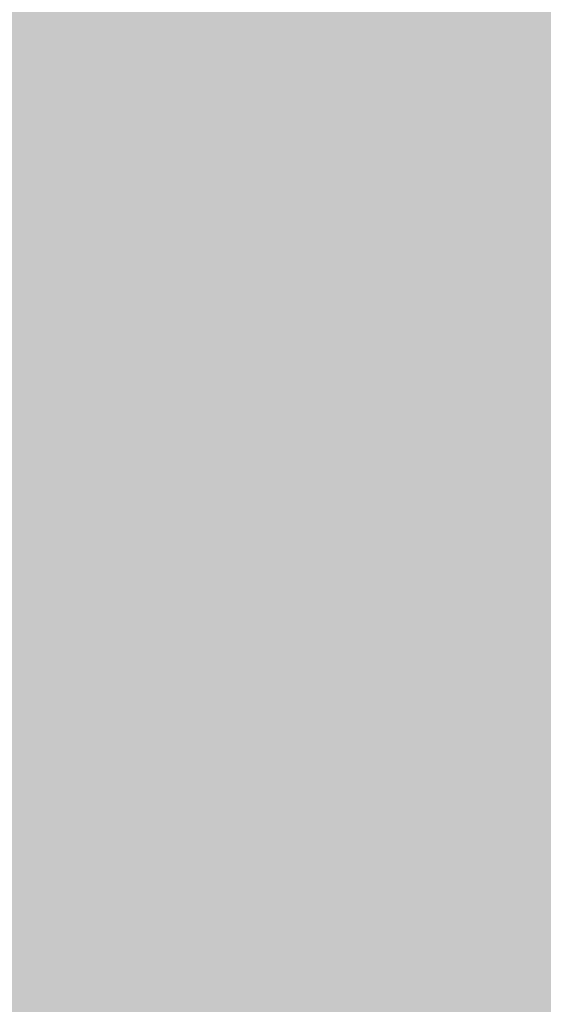
# Model space of a CAD drawing. Units: millimetres. Extents: x -22994 to 29398, y -19990 to 20176.
# Tile 83 of 135: x 227.437 to 229.428, y 79.586 to 83.328. Entities that reach past the tile are written whole.
import ezdxf
from ezdxf import colors
from ezdxf.entities.mleader import LeaderData, LeaderLine
from ezdxf.math import Vec2, Vec3

# ---------------------------------------------------------------- set-up
doc = ezdxf.new("R2010")
doc.units = ezdxf.units.MM
doc.header["$MEASUREMENT"] = 0
doc.layers.add('M-ANNO-TEXT', color=7, linetype='Continuous', lineweight=25)
doc.layers.add('M-DIMS', color=2, linetype='Continuous', lineweight=18)
doc.styles.get("Standard").update_dxf_attribs({"font": 'arial.ttf'})
doc.dimstyles.get("Standard").update_dxf_attribs({"dimtxt": 0.18, "dimasz": 10000, "dimexe": 0.18, "dimexo": 0.0625, "dimgap": 0.09, "dimtad": 0, "dimtih": 1, "dimtoh": 1, "dimdec": 0, "dimzin": 0, "dimdsep": 46, "dimtxsty": 'Standard', "dimcen": 0.09, "dimadec": 0, "dimazin": 0, "dimtfac": 1, "dimtdec": 0, "dimtofl": 0, "dimtmove": 0, "dimatfit": 3, "dimfxl": 1, "dimtolj": 1, "dimtzin": 0, "dimlwd": 30, "dimarcsym": 0})

# ---------------------------------------------------------------- blocks, each defined once
blk = doc.blocks.new('*D2')
at = {"layer": 'Defpoints', "color": 0, "transparency": 16777216}
for p in [(6.6773, 10.2713), (290.852, 10.2713), (290.852, -5.0787)]:
    blk.add_point(p, dxfattribs=at)
at = {"layer": 'M-DIMS', "color": 0, "lineweight": -2, "transparency": 16777216}
for p, q in [((6.6773, 10.2088), (6.6773, -5.2587)), ((290.852, 10.2088), (290.852, -5.2587))]:
    blk.add_line(p, q, dxfattribs=at)
at = {"layer": 'M-DIMS', "color": 0, "lineweight": 30, "transparency": 16777216}
for p, q in [((-9993.3227, -5.0787), (-19993.3227, -5.0787)), ((10290.852, -5.0787), (20290.852, -5.0787))]:
    blk.add_line(p, q, dxfattribs=at)
at = {"layer": 'M-DIMS', "color": 0, "transparency": 16777216}
for points in [[(-9993.3227, 1661.5879), (-9993.3227, -1671.7454), (6.6773, -5.0787)], [(10290.852, 1661.5879), (10290.852, -1671.7454), (290.852, -5.0787)]]:
    blk.add_solid(points, dxfattribs=at)
at = {"layer": 'M-DIMS', "color": 0, "transparency": 16777216, "insert": (148.7647, -5.0787), "char_height": 0.18, "attachment_point": 5}
blk.add_mtext('\\A1;284.2', dxfattribs=at)
blk = doc.blocks.new('*D3')
at = {"layer": 'Defpoints', "color": 0, "transparency": 16777216}
for p in [(110.2647, 204.1654), (110.2647, 176.3662), (95.8327, 127.967)]:
    blk.add_point(p, dxfattribs=at)
at = {"layer": 'M-DIMS', "color": 0, "lineweight": -2, "transparency": 16777216}
for p, q in [((95.8327, 128.0295), (95.8327, 204.3454)), ((110.2647, 176.4287), (110.2647, 204.3454))]:
    blk.add_line(p, q, dxfattribs=at)
at = {"layer": 'M-DIMS', "color": 0, "lineweight": 30, "transparency": 16777216}
for p, q in [((-9904.1673, 204.1654), (-19904.1673, 204.1654)), ((10110.2647, 204.1654), (20110.2647, 204.1654))]:
    blk.add_line(p, q, dxfattribs=at)
at = {"layer": 'M-DIMS', "color": 0, "transparency": 16777216}
for points in [[(-9904.1673, 1870.8321), (-9904.1673, -1462.5013), (95.8327, 204.1654)], [(10110.2647, 1870.8321), (10110.2647, -1462.5013), (110.2647, 204.1654)]]:
    blk.add_solid(points, dxfattribs=at)
at = {"layer": 'M-DIMS', "color": 0, "transparency": 16777216, "insert": (103.0487, 204.1654), "char_height": 0.18, "attachment_point": 5}
blk.add_mtext('\\A1;14.432', dxfattribs=at)
blk = doc.blocks.new('*D4')
at = {"layer": 'Defpoints', "color": 0, "transparency": 16777216}
for p in [(116.2647, 204.1654), (110.2647, 176.3662), (116.2647, 176.3662)]:
    blk.add_point(p, dxfattribs=at)
at = {"layer": 'M-DIMS', "color": 0, "lineweight": -2, "transparency": 16777216}
for p, q in [((110.2647, 176.4287), (110.2647, 204.3454)), ((116.2647, 176.4287), (116.2647, 204.3454))]:
    blk.add_line(p, q, dxfattribs=at)
at = {"layer": 'M-DIMS', "color": 0, "lineweight": 30, "transparency": 16777216}
for p, q in [((-9889.7353, 204.1654), (-19889.7353, 204.1654)), ((10116.2647, 204.1654), (20116.2647, 204.1654))]:
    blk.add_line(p, q, dxfattribs=at)
at = {"layer": 'M-DIMS', "color": 0, "transparency": 16777216}
for points in [[(-9889.7353, 1870.8321), (-9889.7353, -1462.5013), (110.2647, 204.1654)], [(10116.2647, 1870.8321), (10116.2647, -1462.5013), (116.2647, 204.1654)]]:
    blk.add_solid(points, dxfattribs=at)
at = {"layer": 'M-DIMS', "color": 0, "transparency": 16777216, "insert": (113.2647, 204.1654), "char_height": 0.18, "attachment_point": 5}
blk.add_mtext('\\A1;6', dxfattribs=at)
blk = doc.blocks.new('*D5')
at = {"layer": 'Defpoints', "color": 0, "transparency": 16777216}
for p in [(181.2647, 204.1654), (116.2647, 176.3662), (181.2647, 176.3662)]:
    blk.add_point(p, dxfattribs=at)
at = {"layer": 'M-DIMS', "color": 0, "lineweight": -2, "transparency": 16777216}
for p, q in [((116.2647, 176.4287), (116.2647, 204.3454)), ((181.2647, 176.4287), (181.2647, 204.3454))]:
    blk.add_line(p, q, dxfattribs=at)
at = {"layer": 'M-DIMS', "color": 0, "lineweight": 30, "transparency": 16777216}
for p, q in [((-9883.7353, 204.1654), (-19883.7353, 204.1654)), ((10181.2647, 204.1654), (20181.2647, 204.1654))]:
    blk.add_line(p, q, dxfattribs=at)
at = {"layer": 'M-DIMS', "color": 0, "transparency": 16777216}
for points in [[(-9883.7353, 1870.8321), (-9883.7353, -1462.5013), (116.2647, 204.1654)], [(10181.2647, 1870.8321), (10181.2647, -1462.5013), (181.2647, 204.1654)]]:
    blk.add_solid(points, dxfattribs=at)
at = {"layer": 'M-DIMS', "color": 0, "transparency": 16777216, "insert": (148.7647, 204.1654), "char_height": 0.18, "attachment_point": 5}
blk.add_mtext('\\A1;65', dxfattribs=at)
blk = doc.blocks.new('*D6')
at = {"layer": 'Defpoints', "color": 0, "transparency": 16777216}
for p in [(187.2647, 204.1654), (181.2647, 176.3662), (187.2647, 176.3662)]:
    blk.add_point(p, dxfattribs=at)
at = {"layer": 'M-DIMS', "color": 0, "lineweight": -2, "transparency": 16777216}
for p, q in [((181.2647, 176.4287), (181.2647, 204.3454)), ((187.2647, 176.4287), (187.2647, 204.3454))]:
    blk.add_line(p, q, dxfattribs=at)
at = {"layer": 'M-DIMS', "color": 0, "lineweight": 30, "transparency": 16777216}
for p, q in [((-9818.7353, 204.1654), (-19818.7353, 204.1654)), ((10187.2647, 204.1654), (20187.2647, 204.1654))]:
    blk.add_line(p, q, dxfattribs=at)
at = {"layer": 'M-DIMS', "color": 0, "transparency": 16777216}
for points in [[(-9818.7353, 1870.8321), (-9818.7353, -1462.5013), (181.2647, 204.1654)], [(10187.2647, 1870.8321), (10187.2647, -1462.5013), (187.2647, 204.1654)]]:
    blk.add_solid(points, dxfattribs=at)
at = {"layer": 'M-DIMS', "color": 0, "transparency": 16777216, "insert": (184.2647, 204.1654), "char_height": 0.18, "attachment_point": 5}
blk.add_mtext('\\A1;6', dxfattribs=at)
blk = doc.blocks.new('*D7')
at = {"layer": 'Defpoints', "color": 0, "transparency": 16777216}
for p in [(201.6967, 204.1654), (187.2647, 176.3662), (201.6967, 127.967)]:
    blk.add_point(p, dxfattribs=at)
at = {"layer": 'M-DIMS', "color": 0, "lineweight": -2, "transparency": 16777216}
for p, q in [((187.2647, 176.4287), (187.2647, 204.3454)), ((201.6967, 128.0295), (201.6967, 204.3454))]:
    blk.add_line(p, q, dxfattribs=at)
at = {"layer": 'M-DIMS', "color": 0, "lineweight": 30, "transparency": 16777216}
for p, q in [((-9812.7353, 204.1654), (-19812.7353, 204.1654)), ((10201.6967, 204.1654), (20201.6967, 204.1654))]:
    blk.add_line(p, q, dxfattribs=at)
at = {"layer": 'M-DIMS', "color": 0, "transparency": 16777216}
for points in [[(-9812.7353, 1870.8321), (-9812.7353, -1462.5013), (187.2647, 204.1654)], [(10201.6967, 1870.8321), (10201.6967, -1462.5013), (201.6967, 204.1654)]]:
    blk.add_solid(points, dxfattribs=at)
at = {"layer": 'M-DIMS', "color": 0, "transparency": 16777216, "insert": (194.4807, 204.1654), "char_height": 0.18, "attachment_point": 5}
blk.add_mtext('\\A1;14.432', dxfattribs=at)
blk = doc.blocks.new('*D8')
at = {"layer": 'Defpoints', "color": 0, "transparency": 16777216}
for p in [(227.6485, 204.1654), (227.6485, 146.7296), (201.6967, 127.967)]:
    blk.add_point(p, dxfattribs=at)
at = {"layer": 'M-DIMS', "color": 0, "lineweight": -2, "transparency": 16777216}
for p, q in [((201.6967, 128.0295), (201.6967, 204.3454)), ((227.6485, 146.7921), (227.6485, 204.3454))]:
    blk.add_line(p, q, dxfattribs=at)
at = {"layer": 'M-DIMS', "color": 0, "lineweight": 30, "transparency": 16777216}
for p, q in [((-9798.3033, 204.1654), (-19798.3033, 204.1654)), ((10227.6485, 204.1654), (20227.6485, 204.1654))]:
    blk.add_line(p, q, dxfattribs=at)
at = {"layer": 'M-DIMS', "color": 0, "transparency": 16777216}
for points in [[(-9798.3033, 1870.8321), (-9798.3033, -1462.5013), (201.6967, 204.1654)], [(10227.6485, 1870.8321), (10227.6485, -1462.5013), (227.6485, 204.1654)]]:
    blk.add_solid(points, dxfattribs=at)
at = {"layer": 'M-DIMS', "color": 0, "transparency": 16777216, "insert": (214.6726, 204.1654), "char_height": 0.18, "attachment_point": 5}
blk.add_mtext('\\A1;25.95', dxfattribs=at)
blk = doc.blocks.new('*D9')
at = {"layer": 'Defpoints', "color": 0, "transparency": 16777216}
for p in [(187.2647, 176.3662), (306.202, 176.3662), (290.852, 10.2713)]:
    blk.add_point(p, dxfattribs=at)
at = {"layer": 'M-DIMS', "color": 0, "lineweight": 30, "transparency": 16777216}
for p, q in [((306.202, 10176.3662), (306.202, 20176.3662)), ((306.202, -9989.7287), (306.202, -19989.7287))]:
    blk.add_line(p, q, dxfattribs=at)
at = {"layer": 'M-DIMS', "color": 0, "lineweight": -2, "transparency": 16777216}
for p, q in [((187.3272, 176.3662), (306.382, 176.3662)), ((290.9145, 10.2713), (306.382, 10.2713))]:
    blk.add_line(p, q, dxfattribs=at)
at = {"layer": 'M-DIMS', "color": 0, "transparency": 16777216}
for points in [[(-1360.4646, 10176.3662), (1972.8687, 10176.3662), (306.202, 176.3662)], [(-1360.4646, -9989.7287), (1972.8687, -9989.7287), (306.202, 10.2713)]]:
    blk.add_solid(points, dxfattribs=at)
at = {"layer": 'M-DIMS', "color": 0, "transparency": 16777216, "insert": (306.202, 93.3187), "char_height": 0.18, "attachment_point": 5}
blk.add_mtext('\\A1;166.1', dxfattribs=at)
blk = doc.blocks.new('*D10')
at = {"layer": 'Defpoints', "color": 0, "transparency": 16777216}
for p in [(125.6498, 136.0713), (133.3459, 136.0713), (133.3459, -5.0787)]:
    blk.add_point(p, dxfattribs=at)
at = {"layer": 'M-DIMS', "color": 0, "lineweight": -2, "transparency": 16777216}
for p, q in [((125.6498, 136.0088), (125.6498, -5.2587)), ((133.3459, 136.0088), (133.3459, -5.2587))]:
    blk.add_line(p, q, dxfattribs=at)
at = {"layer": 'M-DIMS', "color": 0, "lineweight": 30, "transparency": 16777216}
for p, q in [((-9874.3502, -5.0787), (-19874.3502, -5.0787)), ((10133.3459, -5.0787), (20133.3459, -5.0787))]:
    blk.add_line(p, q, dxfattribs=at)
at = {"layer": 'M-DIMS', "color": 0, "transparency": 16777216}
for points in [[(-9874.3502, 1661.5879), (-9874.3502, -1671.7454), (125.6498, -5.0787)], [(10133.3459, 1661.5879), (10133.3459, -1671.7454), (133.3459, -5.0787)]]:
    blk.add_solid(points, dxfattribs=at)
at = {"layer": 'M-DIMS', "color": 0, "transparency": 16777216, "insert": (129.4978, -5.0787), "char_height": 0.18, "attachment_point": 5}
blk.add_mtext('\\A1;7.696', dxfattribs=at)
blk = doc.blocks.new('*D11')
at = {"layer": 'Defpoints', "color": 0, "transparency": 16777216}
for p in [(133.3459, 136.0713), (135.6498, 136.0713), (135.6498, -5.0787)]:
    blk.add_point(p, dxfattribs=at)
at = {"layer": 'M-DIMS', "color": 0, "lineweight": -2, "transparency": 16777216}
for p, q in [((133.3459, 136.0088), (133.3459, -5.2587)), ((135.6498, 136.0088), (135.6498, -5.2587))]:
    blk.add_line(p, q, dxfattribs=at)
at = {"layer": 'M-DIMS', "color": 0, "lineweight": 30, "transparency": 16777216}
for p, q in [((-9866.6541, -5.0787), (-19866.6541, -5.0787)), ((10135.6498, -5.0787), (20135.6498, -5.0787))]:
    blk.add_line(p, q, dxfattribs=at)
at = {"layer": 'M-DIMS', "color": 0, "transparency": 16777216}
for points in [[(-9866.6541, 1661.5879), (-9866.6541, -1671.7454), (133.3459, -5.0787)], [(10135.6498, 1661.5879), (10135.6498, -1671.7454), (135.6498, -5.0787)]]:
    blk.add_solid(points, dxfattribs=at)
at = {"layer": 'M-DIMS', "color": 0, "transparency": 16777216, "insert": (134.4978, -5.0787), "char_height": 0.18, "attachment_point": 5}
blk.add_mtext('\\A1;2.304', dxfattribs=at)
blk = doc.blocks.new('*D12')
at = {"layer": 'Defpoints', "color": 0, "transparency": 16777216}
for p in [(135.6498, 136.0713), (145.6498, 136.0713), (145.6498, -5.0787)]:
    blk.add_point(p, dxfattribs=at)
at = {"layer": 'M-DIMS', "color": 0, "lineweight": -2, "transparency": 16777216}
for p, q in [((135.6498, 136.0088), (135.6498, -5.2587)), ((145.6498, 136.0088), (145.6498, -5.2587))]:
    blk.add_line(p, q, dxfattribs=at)
at = {"layer": 'M-DIMS', "color": 0, "lineweight": 30, "transparency": 16777216}
for p, q in [((-9864.3502, -5.0787), (-19864.3502, -5.0787)), ((10145.6498, -5.0787), (20145.6498, -5.0787))]:
    blk.add_line(p, q, dxfattribs=at)
at = {"layer": 'M-DIMS', "color": 0, "transparency": 16777216}
for points in [[(-9864.3502, 1661.5879), (-9864.3502, -1671.7454), (135.6498, -5.0787)], [(10145.6498, 1661.5879), (10145.6498, -1671.7454), (145.6498, -5.0787)]]:
    blk.add_solid(points, dxfattribs=at)
at = {"layer": 'M-DIMS', "color": 0, "transparency": 16777216, "insert": (140.6498, -5.0787), "char_height": 0.18, "attachment_point": 5}
blk.add_mtext('\\A1;10', dxfattribs=at)
blk = doc.blocks.new('*D13')
at = {"layer": 'Defpoints', "color": 0, "transparency": 16777216}
for p in [(145.6498, 136.0713), (155.6498, 136.0713), (155.6498, -5.0787)]:
    blk.add_point(p, dxfattribs=at)
at = {"layer": 'M-DIMS', "color": 0, "lineweight": -2, "transparency": 16777216}
for p, q in [((145.6498, 136.0088), (145.6498, -5.2587)), ((155.6498, 136.0088), (155.6498, -5.2587))]:
    blk.add_line(p, q, dxfattribs=at)
at = {"layer": 'M-DIMS', "color": 0, "lineweight": 30, "transparency": 16777216}
for p, q in [((-9854.3502, -5.0787), (-19854.3502, -5.0787)), ((10155.6498, -5.0787), (20155.6498, -5.0787))]:
    blk.add_line(p, q, dxfattribs=at)
at = {"layer": 'M-DIMS', "color": 0, "transparency": 16777216}
for points in [[(-9854.3502, 1661.5879), (-9854.3502, -1671.7454), (145.6498, -5.0787)], [(10155.6498, 1661.5879), (10155.6498, -1671.7454), (155.6498, -5.0787)]]:
    blk.add_solid(points, dxfattribs=at)
at = {"layer": 'M-DIMS', "color": 0, "transparency": 16777216, "insert": (150.6498, -5.0787), "char_height": 0.18, "attachment_point": 5}
blk.add_mtext('\\A1;10', dxfattribs=at)
blk = doc.blocks.new('*D14')
at = {"layer": 'Defpoints', "color": 0, "transparency": 16777216}
for p in [(155.6498, 136.0713), (165.6498, 136.0713), (165.6498, -5.0787)]:
    blk.add_point(p, dxfattribs=at)
at = {"layer": 'M-DIMS', "color": 0, "lineweight": -2, "transparency": 16777216}
for p, q in [((155.6498, 136.0088), (155.6498, -5.2587)), ((165.6498, 136.0088), (165.6498, -5.2587))]:
    blk.add_line(p, q, dxfattribs=at)
at = {"layer": 'M-DIMS', "color": 0, "lineweight": 30, "transparency": 16777216}
for p, q in [((-9844.3502, -5.0787), (-19844.3502, -5.0787)), ((10165.6498, -5.0787), (20165.6498, -5.0787))]:
    blk.add_line(p, q, dxfattribs=at)
at = {"layer": 'M-DIMS', "color": 0, "transparency": 16777216}
for points in [[(-9844.3502, 1661.5879), (-9844.3502, -1671.7454), (155.6498, -5.0787)], [(10165.6498, 1661.5879), (10165.6498, -1671.7454), (165.6498, -5.0787)]]:
    blk.add_solid(points, dxfattribs=at)
at = {"layer": 'M-DIMS', "color": 0, "transparency": 16777216, "insert": (160.6498, -5.0787), "char_height": 0.18, "attachment_point": 5}
blk.add_mtext('\\A1;10', dxfattribs=at)
blk = doc.blocks.new('*D15')
at = {"layer": 'Defpoints', "color": 0, "transparency": 16777216}
for p in [(173.3459, 154.788), (173.3459, 136.0713), (306.202, 136.0713)]:
    blk.add_point(p, dxfattribs=at)
at = {"layer": 'M-DIMS', "color": 0, "lineweight": 30, "transparency": 16777216}
for p, q in [((306.202, 10154.788), (306.202, 20154.788)), ((306.202, -9863.9287), (306.202, -19863.9287))]:
    blk.add_line(p, q, dxfattribs=at)
at = {"layer": 'M-DIMS', "color": 0, "lineweight": -2, "transparency": 16777216}
for p, q in [((173.4084, 154.788), (306.382, 154.788)), ((173.4084, 136.0713), (306.382, 136.0713))]:
    blk.add_line(p, q, dxfattribs=at)
at = {"layer": 'M-DIMS', "color": 0, "transparency": 16777216}
for points in [[(-1360.4646, 10154.788), (1972.8687, 10154.788), (306.202, 154.788)], [(-1360.4646, -9863.9287), (1972.8687, -9863.9287), (306.202, 136.0713)]]:
    blk.add_solid(points, dxfattribs=at)
at = {"layer": 'M-DIMS', "color": 0, "transparency": 16777216, "insert": (306.202, 145.4297), "char_height": 0.18, "attachment_point": 5}
blk.add_mtext('\\A1;18.717', dxfattribs=at)
blk = doc.blocks.new('*D16')
at = {"layer": 'Defpoints', "color": 0, "transparency": 16777216}
for p in [(120.1702, 204.1654), (110.4658, 48.0349), (120.1702, 48.0349)]:
    blk.add_point(p, dxfattribs=at)
at = {"layer": 'M-DIMS', "color": 0, "lineweight": -2, "transparency": 16777216}
for p, q in [((110.4658, 48.0974), (110.4658, 204.3454)), ((120.1702, 48.0974), (120.1702, 204.3454))]:
    blk.add_line(p, q, dxfattribs=at)
at = {"layer": 'M-DIMS', "color": 0, "lineweight": 30, "transparency": 16777216}
for p, q in [((-9889.5342, 204.1654), (-19889.5342, 204.1654)), ((10120.1702, 204.1654), (20120.1702, 204.1654))]:
    blk.add_line(p, q, dxfattribs=at)
at = {"layer": 'M-DIMS', "color": 0, "transparency": 16777216}
for points in [[(-9889.5342, 1870.8321), (-9889.5342, -1462.5013), (110.4658, 204.1654)], [(10120.1702, 1870.8321), (10120.1702, -1462.5013), (120.1702, 204.1654)]]:
    blk.add_solid(points, dxfattribs=at)
at = {"layer": 'M-DIMS', "color": 0, "transparency": 16777216, "insert": (115.318, 204.1654), "char_height": 0.18, "attachment_point": 5}
blk.add_mtext('\\A1;9.704', dxfattribs=at)
blk = doc.blocks.new('*D17')
at = {"layer": 'Defpoints', "color": 0, "transparency": 16777216}
for p in [(126.1702, 204.1654), (120.1702, 48.0349), (126.1702, 48.0349)]:
    blk.add_point(p, dxfattribs=at)
at = {"layer": 'M-DIMS', "color": 0, "lineweight": -2, "transparency": 16777216}
for p, q in [((120.1702, 48.0974), (120.1702, 204.3454)), ((126.1702, 48.0974), (126.1702, 204.3454))]:
    blk.add_line(p, q, dxfattribs=at)
at = {"layer": 'M-DIMS', "color": 0, "lineweight": 30, "transparency": 16777216}
for p, q in [((-9879.8298, 204.1654), (-19879.8298, 204.1654)), ((10126.1702, 204.1654), (20126.1702, 204.1654))]:
    blk.add_line(p, q, dxfattribs=at)
at = {"layer": 'M-DIMS', "color": 0, "transparency": 16777216}
for points in [[(-9879.8298, 1870.8321), (-9879.8298, -1462.5013), (120.1702, 204.1654)], [(10126.1702, 1870.8321), (10126.1702, -1462.5013), (126.1702, 204.1654)]]:
    blk.add_solid(points, dxfattribs=at)
at = {"layer": 'M-DIMS', "color": 0, "transparency": 16777216, "insert": (123.1702, 204.1654), "char_height": 0.18, "attachment_point": 5}
blk.add_mtext('\\A1;6', dxfattribs=at)
blk = doc.blocks.new('*D18')
at = {"layer": 'Defpoints', "color": 0, "transparency": 16777216}
for p in [(132.1702, 204.1654), (126.1702, 48.0349), (132.1702, 48.0349)]:
    blk.add_point(p, dxfattribs=at)
at = {"layer": 'M-DIMS', "color": 0, "lineweight": -2, "transparency": 16777216}
for p, q in [((126.1702, 48.0974), (126.1702, 204.3454)), ((132.1702, 48.0974), (132.1702, 204.3454))]:
    blk.add_line(p, q, dxfattribs=at)
at = {"layer": 'M-DIMS', "color": 0, "lineweight": 30, "transparency": 16777216}
for p, q in [((-9873.8298, 204.1654), (-19873.8298, 204.1654)), ((10132.1702, 204.1654), (20132.1702, 204.1654))]:
    blk.add_line(p, q, dxfattribs=at)
at = {"layer": 'M-DIMS', "color": 0, "transparency": 16777216}
for points in [[(-9873.8298, 1870.8321), (-9873.8298, -1462.5013), (126.1702, 204.1654)], [(10132.1702, 1870.8321), (10132.1702, -1462.5013), (132.1702, 204.1654)]]:
    blk.add_solid(points, dxfattribs=at)
at = {"layer": 'M-DIMS', "color": 0, "transparency": 16777216, "insert": (129.1702, 204.1654), "char_height": 0.18, "attachment_point": 5}
blk.add_mtext('\\A1;6', dxfattribs=at)
blk = doc.blocks.new('*D19')
at = {"layer": 'Defpoints', "color": 0, "transparency": 16777216}
for p in [(138.1702, 204.1654), (132.1702, 48.0349), (138.1702, 48.0349)]:
    blk.add_point(p, dxfattribs=at)
at = {"layer": 'M-DIMS', "color": 0, "lineweight": -2, "transparency": 16777216}
for p, q in [((132.1702, 48.0974), (132.1702, 204.3454)), ((138.1702, 48.0974), (138.1702, 204.3454))]:
    blk.add_line(p, q, dxfattribs=at)
at = {"layer": 'M-DIMS', "color": 0, "lineweight": 30, "transparency": 16777216}
for p, q in [((-9867.8298, 204.1654), (-19867.8298, 204.1654)), ((10138.1702, 204.1654), (20138.1702, 204.1654))]:
    blk.add_line(p, q, dxfattribs=at)
at = {"layer": 'M-DIMS', "color": 0, "transparency": 16777216}
for points in [[(-9867.8298, 1870.8321), (-9867.8298, -1462.5013), (132.1702, 204.1654)], [(10138.1702, 1870.8321), (10138.1702, -1462.5013), (138.1702, 204.1654)]]:
    blk.add_solid(points, dxfattribs=at)
at = {"layer": 'M-DIMS', "color": 0, "transparency": 16777216, "insert": (135.1702, 204.1654), "char_height": 0.18, "attachment_point": 5}
blk.add_mtext('\\A1;6', dxfattribs=at)
blk = doc.blocks.new('*D20')
at = {"layer": 'Defpoints', "color": 0, "transparency": 16777216}
for p in [(144.1702, 204.1654), (138.1702, 48.0349), (144.1702, 48.0349)]:
    blk.add_point(p, dxfattribs=at)
at = {"layer": 'M-DIMS', "color": 0, "lineweight": -2, "transparency": 16777216}
for p, q in [((138.1702, 48.0974), (138.1702, 204.3454)), ((144.1702, 48.0974), (144.1702, 204.3454))]:
    blk.add_line(p, q, dxfattribs=at)
at = {"layer": 'M-DIMS', "color": 0, "lineweight": 30, "transparency": 16777216}
for p, q in [((-9861.8298, 204.1654), (-19861.8298, 204.1654)), ((10144.1702, 204.1654), (20144.1702, 204.1654))]:
    blk.add_line(p, q, dxfattribs=at)
at = {"layer": 'M-DIMS', "color": 0, "transparency": 16777216}
for points in [[(-9861.8298, 1870.8321), (-9861.8298, -1462.5013), (138.1702, 204.1654)], [(10144.1702, 1870.8321), (10144.1702, -1462.5013), (144.1702, 204.1654)]]:
    blk.add_solid(points, dxfattribs=at)
at = {"layer": 'M-DIMS', "color": 0, "transparency": 16777216, "insert": (141.1702, 204.1654), "char_height": 0.18, "attachment_point": 5}
blk.add_mtext('\\A1;6', dxfattribs=at)
blk = doc.blocks.new('*D21')
at = {"layer": 'Defpoints', "color": 0, "transparency": 16777216}
for p in [(149.1157, 204.1654), (144.1702, 48.0349), (149.1157, 48.0349)]:
    blk.add_point(p, dxfattribs=at)
at = {"layer": 'M-DIMS', "color": 0, "lineweight": -2, "transparency": 16777216}
for p, q in [((144.1702, 48.0974), (144.1702, 204.3454)), ((149.1157, 48.0974), (149.1157, 204.3454))]:
    blk.add_line(p, q, dxfattribs=at)
at = {"layer": 'M-DIMS', "color": 0, "lineweight": 30, "transparency": 16777216}
for p, q in [((-9855.8298, 204.1654), (-19855.8298, 204.1654)), ((10149.1157, 204.1654), (20149.1157, 204.1654))]:
    blk.add_line(p, q, dxfattribs=at)
at = {"layer": 'M-DIMS', "color": 0, "transparency": 16777216}
for points in [[(-9855.8298, 1870.8321), (-9855.8298, -1462.5013), (144.1702, 204.1654)], [(10149.1157, 1870.8321), (10149.1157, -1462.5013), (149.1157, 204.1654)]]:
    blk.add_solid(points, dxfattribs=at)
at = {"layer": 'M-DIMS', "color": 0, "transparency": 16777216, "insert": (146.6429, 204.1654), "char_height": 0.18, "attachment_point": 5}
blk.add_mtext('\\A1;4.945', dxfattribs=at)
blk = doc.blocks.new('*D22')
at = {"layer": 'Defpoints', "color": 0, "transparency": 16777216}
for p in [(149.1157, 30.9895), (155.1157, 30.9895), (155.1157, -5.0787)]:
    blk.add_point(p, dxfattribs=at)
at = {"layer": 'M-DIMS', "color": 0, "lineweight": -2, "transparency": 16777216}
for p, q in [((149.1157, 30.927), (149.1157, -5.2587)), ((155.1157, 30.927), (155.1157, -5.2587))]:
    blk.add_line(p, q, dxfattribs=at)
at = {"layer": 'M-DIMS', "color": 0, "lineweight": 30, "transparency": 16777216}
for p, q in [((-9850.8843, -5.0787), (-19850.8843, -5.0787)), ((10155.1157, -5.0787), (20155.1157, -5.0787))]:
    blk.add_line(p, q, dxfattribs=at)
at = {"layer": 'M-DIMS', "color": 0, "transparency": 16777216}
for points in [[(-9850.8843, 1661.5879), (-9850.8843, -1671.7454), (149.1157, -5.0787)], [(10155.1157, 1661.5879), (10155.1157, -1671.7454), (155.1157, -5.0787)]]:
    blk.add_solid(points, dxfattribs=at)
at = {"layer": 'M-DIMS', "color": 0, "transparency": 16777216, "insert": (152.1157, -5.0787), "char_height": 0.18, "attachment_point": 5}
blk.add_mtext('\\A1;6', dxfattribs=at)
blk = doc.blocks.new('*D23')
at = {"layer": 'Defpoints', "color": 0, "transparency": 16777216}
for p in [(155.1157, 30.9895), (161.1157, 30.9895), (161.1157, -5.0787)]:
    blk.add_point(p, dxfattribs=at)
at = {"layer": 'M-DIMS', "color": 0, "lineweight": -2, "transparency": 16777216}
for p, q in [((155.1157, 30.927), (155.1157, -5.2587)), ((161.1157, 30.927), (161.1157, -5.2587))]:
    blk.add_line(p, q, dxfattribs=at)
at = {"layer": 'M-DIMS', "color": 0, "lineweight": 30, "transparency": 16777216}
for p, q in [((-9844.8843, -5.0787), (-19844.8843, -5.0787)), ((10161.1157, -5.0787), (20161.1157, -5.0787))]:
    blk.add_line(p, q, dxfattribs=at)
at = {"layer": 'M-DIMS', "color": 0, "transparency": 16777216}
for points in [[(-9844.8843, 1661.5879), (-9844.8843, -1671.7454), (155.1157, -5.0787)], [(10161.1157, 1661.5879), (10161.1157, -1671.7454), (161.1157, -5.0787)]]:
    blk.add_solid(points, dxfattribs=at)
at = {"layer": 'M-DIMS', "color": 0, "transparency": 16777216, "insert": (158.1157, -5.0787), "char_height": 0.18, "attachment_point": 5}
blk.add_mtext('\\A1;6', dxfattribs=at)
blk = doc.blocks.new('*D24')
at = {"layer": 'Defpoints', "color": 0, "transparency": 16777216}
for p in [(161.1157, 30.9895), (166.4387, 30.9895), (166.4387, -5.0787)]:
    blk.add_point(p, dxfattribs=at)
at = {"layer": 'M-DIMS', "color": 0, "lineweight": -2, "transparency": 16777216}
for p, q in [((161.1157, 30.927), (161.1157, -5.2587)), ((166.4387, 30.927), (166.4387, -5.2587))]:
    blk.add_line(p, q, dxfattribs=at)
at = {"layer": 'M-DIMS', "color": 0, "lineweight": 30, "transparency": 16777216}
for p, q in [((-9838.8843, -5.0787), (-19838.8843, -5.0787)), ((10166.4387, -5.0787), (20166.4387, -5.0787))]:
    blk.add_line(p, q, dxfattribs=at)
at = {"layer": 'M-DIMS', "color": 0, "transparency": 16777216}
for points in [[(-9838.8843, 1661.5879), (-9838.8843, -1671.7454), (161.1157, -5.0787)], [(10166.4387, 1661.5879), (10166.4387, -1671.7454), (166.4387, -5.0787)]]:
    blk.add_solid(points, dxfattribs=at)
at = {"layer": 'M-DIMS', "color": 0, "transparency": 16777216, "insert": (163.7772, -5.0787), "char_height": 0.18, "attachment_point": 5}
blk.add_mtext('\\A1;5.323', dxfattribs=at)
blk = doc.blocks.new('*D25')
at = {"layer": 'Defpoints', "color": 0, "transparency": 16777216}
for p in [(166.4387, 30.9895), (172.4387, 30.9895), (172.4387, -5.0787)]:
    blk.add_point(p, dxfattribs=at)
at = {"layer": 'M-DIMS', "color": 0, "lineweight": -2, "transparency": 16777216}
for p, q in [((166.4387, 30.927), (166.4387, -5.2587)), ((172.4387, 30.927), (172.4387, -5.2587))]:
    blk.add_line(p, q, dxfattribs=at)
at = {"layer": 'M-DIMS', "color": 0, "lineweight": 30, "transparency": 16777216}
for p, q in [((-9833.5613, -5.0787), (-19833.5613, -5.0787)), ((10172.4387, -5.0787), (20172.4387, -5.0787))]:
    blk.add_line(p, q, dxfattribs=at)
at = {"layer": 'M-DIMS', "color": 0, "transparency": 16777216}
for points in [[(-9833.5613, 1661.5879), (-9833.5613, -1671.7454), (166.4387, -5.0787)], [(10172.4387, 1661.5879), (10172.4387, -1671.7454), (172.4387, -5.0787)]]:
    blk.add_solid(points, dxfattribs=at)
at = {"layer": 'M-DIMS', "color": 0, "transparency": 16777216, "insert": (169.4387, -5.0787), "char_height": 0.18, "attachment_point": 5}
blk.add_mtext('\\A1;6', dxfattribs=at)
blk = doc.blocks.new('*D26')
at = {"layer": 'Defpoints', "color": 0, "transparency": 16777216}
for p in [(172.4387, 30.9895), (178.4387, 30.9895), (178.4387, -5.0787)]:
    blk.add_point(p, dxfattribs=at)
at = {"layer": 'M-DIMS', "color": 0, "lineweight": -2, "transparency": 16777216}
for p, q in [((172.4387, 30.927), (172.4387, -5.2587)), ((178.4387, 30.927), (178.4387, -5.2587))]:
    blk.add_line(p, q, dxfattribs=at)
at = {"layer": 'M-DIMS', "color": 0, "lineweight": 30, "transparency": 16777216}
for p, q in [((-9827.5613, -5.0787), (-19827.5613, -5.0787)), ((10178.4387, -5.0787), (20178.4387, -5.0787))]:
    blk.add_line(p, q, dxfattribs=at)
at = {"layer": 'M-DIMS', "color": 0, "transparency": 16777216}
for points in [[(-9827.5613, 1661.5879), (-9827.5613, -1671.7454), (172.4387, -5.0787)], [(10178.4387, 1661.5879), (10178.4387, -1671.7454), (178.4387, -5.0787)]]:
    blk.add_solid(points, dxfattribs=at)
at = {"layer": 'M-DIMS', "color": 0, "transparency": 16777216, "insert": (175.4387, -5.0787), "char_height": 0.18, "attachment_point": 5}
blk.add_mtext('\\A1;6', dxfattribs=at)
blk = doc.blocks.new('*D27')
at = {"layer": 'Defpoints', "color": 0, "transparency": 16777216}
for p in [(178.4387, 30.9895), (188.1175, 30.9895), (188.1175, -5.0787)]:
    blk.add_point(p, dxfattribs=at)
at = {"layer": 'M-DIMS', "color": 0, "lineweight": -2, "transparency": 16777216}
for p, q in [((178.4387, 30.927), (178.4387, -5.2587)), ((188.1175, 30.927), (188.1175, -5.2587))]:
    blk.add_line(p, q, dxfattribs=at)
at = {"layer": 'M-DIMS', "color": 0, "lineweight": 30, "transparency": 16777216}
for p, q in [((-9821.5613, -5.0787), (-19821.5613, -5.0787)), ((10188.1175, -5.0787), (20188.1175, -5.0787))]:
    blk.add_line(p, q, dxfattribs=at)
at = {"layer": 'M-DIMS', "color": 0, "transparency": 16777216}
for points in [[(-9821.5613, 1661.5879), (-9821.5613, -1671.7454), (178.4387, -5.0787)], [(10188.1175, 1661.5879), (10188.1175, -1671.7454), (188.1175, -5.0787)]]:
    blk.add_solid(points, dxfattribs=at)
at = {"layer": 'M-DIMS', "color": 0, "transparency": 16777216, "insert": (183.2781, -5.0787), "char_height": 0.18, "attachment_point": 5}
blk.add_mtext('\\A1;9.679', dxfattribs=at)
blk = doc.blocks.new('*D28')
at = {"layer": 'Defpoints', "color": 0, "transparency": 16777216}
for p in [(188.1175, 48.0349), (306.202, 48.0349), (188.1175, 30.9895)]:
    blk.add_point(p, dxfattribs=at)
at = {"layer": 'M-DIMS', "color": 0, "lineweight": 30, "transparency": 16777216}
for p, q in [((306.202, 10048.0349), (306.202, 20048.0349)), ((306.202, -9969.0105), (306.202, -19969.0105))]:
    blk.add_line(p, q, dxfattribs=at)
at = {"layer": 'M-DIMS', "color": 0, "lineweight": -2, "transparency": 16777216}
for p, q in [((188.18, 48.0349), (306.382, 48.0349)), ((188.18, 30.9895), (306.382, 30.9895))]:
    blk.add_line(p, q, dxfattribs=at)
at = {"layer": 'M-DIMS', "color": 0, "transparency": 16777216}
for points in [[(-1360.4646, 10048.0349), (1972.8687, 10048.0349), (306.202, 48.0349)], [(-1360.4646, -9969.0105), (1972.8687, -9969.0105), (306.202, 30.9895)]]:
    blk.add_solid(points, dxfattribs=at)
at = {"layer": 'M-DIMS', "color": 0, "transparency": 16777216, "insert": (306.202, 39.5122), "char_height": 0.18, "attachment_point": 5}
blk.add_mtext('\\A1;17.045', dxfattribs=at)
blk = doc.blocks.new('*D29')
at = {"layer": 'Defpoints', "color": 0, "transparency": 16777216}
for p in [(36.8006, 80.045), (64.0296, 80.045)]:
    blk.add_point(p, dxfattribs=at)
at = {"layer": 'M-DIMS', "color": 0, "lineweight": -2, "transparency": 16777216}
for p, q in [((50.4151, 79.955), (50.4151, 80.135)), ((50.3251, 80.045), (50.5051, 80.045))]:
    blk.add_line(p, q, dxfattribs=at)
at = {"layer": 'M-DIMS', "color": 0, "lineweight": 30, "transparency": 16777216}
blk.add_line((20064.0296, 80.0303), (10064.0296, 80.0377), dxfattribs=at)
at = {"layer": 'M-DIMS', "color": 0, "transparency": 16777216}
blk.add_solid([(10064.0309, 1746.7043), (10064.0284, -1586.629), (64.0296, 80.045)], dxfattribs=at)
at = {"layer": 'M-DIMS', "color": 0, "transparency": 16777216, "insert": (20064.5213, 80.0303), "char_height": 0.18, "attachment_point": 5}
blk.add_mtext('\\A1;∅27.23', dxfattribs=at)
blk = doc.blocks.new('*D30')
at = {"layer": 'Defpoints', "color": 0, "transparency": 16777216}
for p in [(216.3148, 146.7291), (238.9821, 146.73)]:
    blk.add_point(p, dxfattribs=at)
at = {"layer": 'M-DIMS', "color": 0, "lineweight": 30, "transparency": 16777216}
blk.add_line((20238.9821, 147.4959), (10238.9821, 147.1129), dxfattribs=at)
at = {"layer": 'M-DIMS', "color": 0, "lineweight": -2, "transparency": 16777216}
for p, q in [((227.6485, 146.6396), (227.6485, 146.8196)), ((227.5585, 146.7296), (227.7385, 146.7296))]:
    blk.add_line(p, q, dxfattribs=at)
at = {"layer": 'M-DIMS', "color": 0, "transparency": 16777216}
blk.add_solid([(10238.9183, 1813.7796), (10239.0459, -1519.5537), (238.9821, 146.73)], dxfattribs=at)
at = {"layer": 'M-DIMS', "color": 0, "transparency": 16777216, "insert": (20239.5436, 147.4959), "char_height": 0.18, "attachment_point": 5}
blk.add_mtext('\\A1;∅22.667', dxfattribs=at)
blk = doc.blocks.new('*D31')
at = {"layer": 'Defpoints', "color": 0, "transparency": 16777216}
for p in [(223.1641, 146.7291), (232.1328, 146.73)]:
    blk.add_point(p, dxfattribs=at)
at = {"layer": 'M-DIMS', "color": 0, "lineweight": 30, "transparency": 16777216}
blk.add_line((20232.1327, 148.6656), (10232.1328, 147.6978), dxfattribs=at)
at = {"layer": 'M-DIMS', "color": 0, "lineweight": -2, "transparency": 16777216}
for p, q in [((227.6485, 146.6396), (227.6485, 146.8196)), ((227.5585, 146.7296), (227.7385, 146.7296))]:
    blk.add_line(p, q, dxfattribs=at)
at = {"layer": 'M-DIMS', "color": 0, "transparency": 16777216}
blk.add_solid([(10231.9715, 1814.3645), (10232.2941, -1518.9688), (232.1328, 146.73)], dxfattribs=at)
at = {"layer": 'M-DIMS', "color": 0, "transparency": 16777216, "insert": (20232.6245, 148.6656), "char_height": 0.18, "attachment_point": 5}
blk.add_mtext('\\A1;∅8.969', dxfattribs=at)
blk = doc.blocks.new('*D36')
at = {"layer": 'Defpoints', "color": 0, "transparency": 16777216}
for p in [(46.39, 31.3035), (46.3875, 26.5934)]:
    blk.add_point(p, dxfattribs=at)
at = {"layer": 'M-DIMS', "color": 0, "lineweight": 30, "transparency": 16777216}
for p, q in [((57.1499, 20031.3006), (51.77, 10031.302)), ((10057.1499, 20031.3006), (57.1499, 20031.3006))]:
    blk.add_line(p, q, dxfattribs=at)
at = {"layer": 'M-DIMS', "color": 0, "lineweight": -2, "transparency": 16777216}
for p, q in [((46.3887, 28.8585), (46.3887, 29.0385)), ((46.2987, 28.9485), (46.4787, 28.9485))]:
    blk.add_line(p, q, dxfattribs=at)
at = {"layer": 'M-DIMS', "color": 0, "transparency": 16777216}
blk.add_solid([(-1614.8965, 10032.1987), (1718.4364, 10030.4054), (46.39, 31.3035)], dxfattribs=at)
at = {"layer": 'M-DIMS', "color": 0, "transparency": 16777216, "insert": (10057.5542, 20031.3006), "char_height": 0.18, "attachment_point": 5}
blk.add_mtext('\\A1;∅4.71', dxfattribs=at)
blk = doc.blocks.new('*D37')
at = {"layer": 'Defpoints', "color": 0, "transparency": 16777216}
for p in [(54.8343, 118.6145), (59.4936, 118.614)]:
    blk.add_point(p, dxfattribs=at)
at = {"layer": 'M-DIMS', "color": 0, "lineweight": -2, "transparency": 16777216}
for p, q in [((57.1639, 118.5243), (57.1639, 118.7043)), ((57.0739, 118.6143), (57.2539, 118.6143))]:
    blk.add_line(p, q, dxfattribs=at)
at = {"layer": 'M-DIMS', "color": 0, "lineweight": 30, "transparency": 16777216}
blk.add_line((20059.4934, 116.2531), (10059.4935, 117.4336), dxfattribs=at)
at = {"layer": 'M-DIMS', "color": 0, "transparency": 16777216}
blk.add_solid([(10059.6902, 1784.1002), (10059.2968, -1549.2331), (59.4936, 118.614)], dxfattribs=at)
at = {"layer": 'M-DIMS', "color": 0, "transparency": 16777216, "insert": (20059.9852, 116.2531), "char_height": 0.18, "attachment_point": 5}
blk.add_mtext('\\A1;∅4.659', dxfattribs=at)

msp = doc.modelspace()

# ---------------------------------------------------------------- dimensions: what is measured, and where the dimension line sits
at = {"layer": 'M-DIMS'}
for base, p1, p2, override, picture, middle in [((306.202, 176.3662), (290.852, 10.2713), (187.2647, 176.3662), {"dimdec": 1, "dimlfac": 1, "dimrnd": 0, "dimzin": 0, "dimdsep": 46, "dimlunit": 2}, '*D9', (306.202, 93.3187)), ((306.202, 136.0713), (173.3459, 154.788), (173.3459, 136.0713), {"dimdec": 3, "dimlfac": 1, "dimrnd": 0, "dimzin": 0, "dimdsep": 46, "dimlunit": 2}, '*D15', (306.202, 145.4297)), ((306.202, 48.0349), (188.1175, 30.9895), (188.1175, 48.0349), {"dimdec": 3, "dimlfac": 1, "dimrnd": 0, "dimzin": 0, "dimdsep": 46, "dimlunit": 2}, '*D28', (306.202, 39.5122))]:
    dim = msp.add_linear_dim(base=base, p1=p1, p2=p2, angle=90, dimstyle='Standard', override=override, dxfattribs=at)
    dim.commit()
    dim.dimension.update_dxf_attribs({"geometry": picture, "text_midpoint": middle})
for p1, p2, override, picture, middle in [((46.3875, 26.5934), (46.39, 31.3035), {"dimdec": 2, "dimlfac": 1, "dimrnd": 0, "dimzin": 0, "dimdsep": 46, "dimlunit": 2}, '*D36', (10057.5542, 20031.3006)), ((223.1641, 146.7291), (232.1328, 146.73), {"dimdec": 3, "dimlfac": 1, "dimrnd": 0, "dimzin": 0, "dimdsep": 46, "dimlunit": 2}, '*D31', (20232.1327, 148.6656)), ((216.3148, 146.7291), (238.9821, 146.73), {"dimdec": 3, "dimlfac": 1, "dimrnd": 0, "dimzin": 0, "dimdsep": 46, "dimlunit": 2}, '*D30', (20238.9821, 147.4959))]:
    dim = msp.add_diameter_dim_2p(p1=p1, p2=p2, dimstyle='Standard', override=override, dxfattribs=at)
    dim.commit()
    dim.dimension.update_dxf_attribs({"geometry": picture, "text_midpoint": middle, "dimtype": 163})
for base, p1, p2, override, picture, middle in [((110.2647, 204.1654), (95.8327, 127.967), (110.2647, 176.3662), {"dimdec": 3, "dimlfac": 1, "dimrnd": 0, "dimzin": 0, "dimdsep": 46, "dimlunit": 2}, '*D3', (103.0487, 204.1654)), ((116.2647, 204.1654), (110.2647, 176.3662), (116.2647, 176.3662), {"dimdec": 0, "dimlfac": 1, "dimrnd": 0, "dimzin": 0, "dimdsep": 46, "dimlunit": 2}, '*D4', (113.2647, 204.1654)), ((120.1702, 204.1654), (110.4658, 48.0349), (120.1702, 48.0349), {"dimdec": 3, "dimlfac": 1, "dimrnd": 0, "dimzin": 0, "dimdsep": 46, "dimlunit": 2}, '*D16', (115.318, 204.1654)), ((181.2647, 204.1654), (116.2647, 176.3662), (181.2647, 176.3662), {"dimdec": 0, "dimlfac": 1, "dimrnd": 0, "dimzin": 0, "dimdsep": 46, "dimlunit": 2}, '*D5', (148.7647, 204.1654)), ((126.1702, 204.1654), (120.1702, 48.0349), (126.1702, 48.0349), {"dimdec": 0, "dimlfac": 1, "dimrnd": 0, "dimzin": 0, "dimdsep": 46, "dimlunit": 2}, '*D17', (123.1702, 204.1654)), ((132.1702, 204.1654), (126.1702, 48.0349), (132.1702, 48.0349), {"dimdec": 0, "dimlfac": 1, "dimrnd": 0, "dimzin": 0, "dimdsep": 46, "dimlunit": 2}, '*D18', (129.1702, 204.1654)), ((138.1702, 204.1654), (132.1702, 48.0349), (138.1702, 48.0349), {"dimdec": 0, "dimlfac": 1, "dimrnd": 0, "dimzin": 0, "dimdsep": 46, "dimlunit": 2}, '*D19', (135.1702, 204.1654)), ((144.1702, 204.1654), (138.1702, 48.0349), (144.1702, 48.0349), {"dimdec": 0, "dimlfac": 1, "dimrnd": 0, "dimzin": 0, "dimdsep": 46, "dimlunit": 2}, '*D20', (141.1702, 204.1654)), ((149.11567, 204.16539), (144.17023, 48.03494), (149.11567, 48.03494), {"dimdec": 3, "dimlfac": 1, "dimrnd": 0, "dimzin": 0, "dimdsep": 46, "dimlunit": 2}, '*D21', (146.64295, 204.16539)), ((187.2647, 204.1654), (181.2647, 176.3662), (187.2647, 176.3662), {"dimdec": 0, "dimlfac": 1, "dimrnd": 0, "dimzin": 0, "dimdsep": 46, "dimlunit": 2}, '*D6', (184.2647, 204.1654)), ((201.6967, 204.1654), (187.2647, 176.3662), (201.6967, 127.967), {"dimdec": 3, "dimlfac": 1, "dimrnd": 0, "dimzin": 0, "dimdsep": 46, "dimlunit": 2}, '*D7', (194.4807, 204.1654)), ((227.6485, 204.1654), (201.6967, 127.967), (227.6485, 146.7296), {"dimdec": 2, "dimlfac": 1, "dimrnd": 0, "dimzin": 0, "dimdsep": 46, "dimlunit": 2}, '*D8', (214.6726, 204.1654)), ((290.852, -5.0787), (6.6773, 10.2713), (290.852, 10.2713), {"dimdec": 1, "dimlfac": 1, "dimrnd": 0, "dimzin": 0, "dimdsep": 46, "dimlunit": 2}, '*D2', (148.7647, -5.0787)), ((133.3459, -5.0787), (125.6498, 136.0713), (133.3459, 136.0713), {"dimdec": 3, "dimlfac": 1, "dimrnd": 0, "dimzin": 0, "dimdsep": 46, "dimlunit": 2}, '*D10', (129.4978, -5.0787)), ((135.6498, -5.0787), (133.3459, 136.0713), (135.6498, 136.0713), {"dimdec": 3, "dimlfac": 1, "dimrnd": 0, "dimzin": 0, "dimdsep": 46, "dimlunit": 2}, '*D11', (134.4978, -5.0787)), ((145.6498, -5.0787), (135.6498, 136.0713), (145.6498, 136.0713), {"dimdec": 0, "dimlfac": 1, "dimrnd": 0, "dimzin": 0, "dimdsep": 46, "dimlunit": 2}, '*D12', (140.6498, -5.0787)), ((155.6498, -5.0787), (145.6498, 136.0713), (155.6498, 136.0713), {"dimdec": 0, "dimlfac": 1, "dimrnd": 0, "dimzin": 0, "dimdsep": 46, "dimlunit": 2}, '*D13', (150.6498, -5.0787)), ((155.1157, -5.0787), (149.1157, 30.9895), (155.1157, 30.9895), {"dimdec": 0, "dimlfac": 1, "dimrnd": 0, "dimzin": 0, "dimdsep": 46, "dimlunit": 2}, '*D22', (152.1157, -5.0787)), ((161.1157, -5.0787), (155.1157, 30.9895), (161.1157, 30.9895), {"dimdec": 0, "dimlfac": 1, "dimrnd": 0, "dimzin": 0, "dimdsep": 46, "dimlunit": 2}, '*D23', (158.1157, -5.0787)), ((165.6498, -5.0787), (155.6498, 136.0713), (165.6498, 136.0713), {"dimdec": 0, "dimlfac": 1, "dimrnd": 0, "dimzin": 0, "dimdsep": 46, "dimlunit": 2}, '*D14', (160.6498, -5.0787)), ((166.4387, -5.0787), (161.1157, 30.9895), (166.4387, 30.9895), {"dimdec": 3, "dimlfac": 1, "dimrnd": 0, "dimzin": 0, "dimdsep": 46, "dimlunit": 2}, '*D24', (163.7772, -5.0787)), ((172.4387, -5.0787), (166.4387, 30.9895), (172.4387, 30.9895), {"dimdec": 0, "dimlfac": 1, "dimrnd": 0, "dimzin": 0, "dimdsep": 46, "dimlunit": 2}, '*D25', (169.4387, -5.0787)), ((178.4387, -5.0787), (172.4387, 30.9895), (178.4387, 30.9895), {"dimdec": 0, "dimlfac": 1, "dimrnd": 0, "dimzin": 0, "dimdsep": 46, "dimlunit": 2}, '*D26', (175.4387, -5.0787)), ((188.1175, -5.0787), (178.4387, 30.9895), (188.1175, 30.9895), {"dimdec": 3, "dimlfac": 1, "dimrnd": 0, "dimzin": 0, "dimdsep": 46, "dimlunit": 2}, '*D27', (183.2781, -5.0787))]:
    dim = msp.add_linear_dim(base=base, p1=p1, p2=p2, dimstyle='Standard', override=override, dxfattribs=at)
    dim.commit()
    dim.dimension.update_dxf_attribs({"geometry": picture, "text_midpoint": middle})
for p1, p2, override, picture, middle in [((54.8343, 118.6145), (59.4936, 118.614), {"dimdec": 3, "dimlfac": 1, "dimrnd": 0, "dimzin": 0, "dimdsep": 46, "dimlunit": 2}, '*D37', (20059.4934, 116.2531)), ((36.8006, 80.045), (64.0296, 80.045), {"dimdec": 2, "dimlfac": 1, "dimrnd": 0, "dimzin": 0, "dimdsep": 46, "dimlunit": 2}, '*D29', (20064.0296, 80.0303))]:
    dim = msp.add_diameter_dim_2p(p1=p1, p2=p2, dimstyle='Standard', override=override, dxfattribs=at)
    dim.commit()
    dim.dimension.update_dxf_attribs({"geometry": picture, "text_midpoint": middle})

# ---------------------------------------------------------------- leaders
at = {"layer": 'M-ANNO-TEXT'}
ml = msp.add_multileader_mtext('Standard', dxfattribs=at)
ml.set_content('combustion chamber', color=256)
ml.set_leader_properties()
ml.build(insert=Vec2(0, 0))
ml.multileader.update_dxf_attribs({"dogleg_length": 0.36, "arrow_head_size": 200})
ctx = ml.context
ctx.base_point, ctx.char_height, ctx.arrow_head_size, ctx.landing_gap_size, ctx.plane_origin = Vec3(215.7321, 57.9149), 3, 200, 0.09, Vec3(189.1175, 57.9149)
notes = []
notes.append((ctx, [(0, (1, 1, 0), (215.3721, 57.9149), (1, 0), 0.36, [(0, [(189.1175, 57.9149)], 0, [])])]))
ctx.mtext.insert, ctx.mtext.flow_direction = Vec3(215.8221, 59.4394), 5
for ctx, leaders in notes:
    for number, flags, end, landing, length, lines in leaders:
        leader = LeaderData()
        leader.index, (leader.has_last_leader_line, leader.has_dogleg_vector, leader.attachment_direction) = number, flags
        leader.last_leader_point, leader.dogleg_vector, leader.dogleg_length = Vec3(end), Vec3(landing), length
        for number, points, colour, breaks in lines:
            line = LeaderLine()
            line.index, line.vertices, line.color, line.breaks = number, Vec3.list(points), colors.encode_raw_color(colour), breaks
            leader.lines.append(line)
        ctx.leaders.append(leader)

doc.saveas('drawing.dxf')
